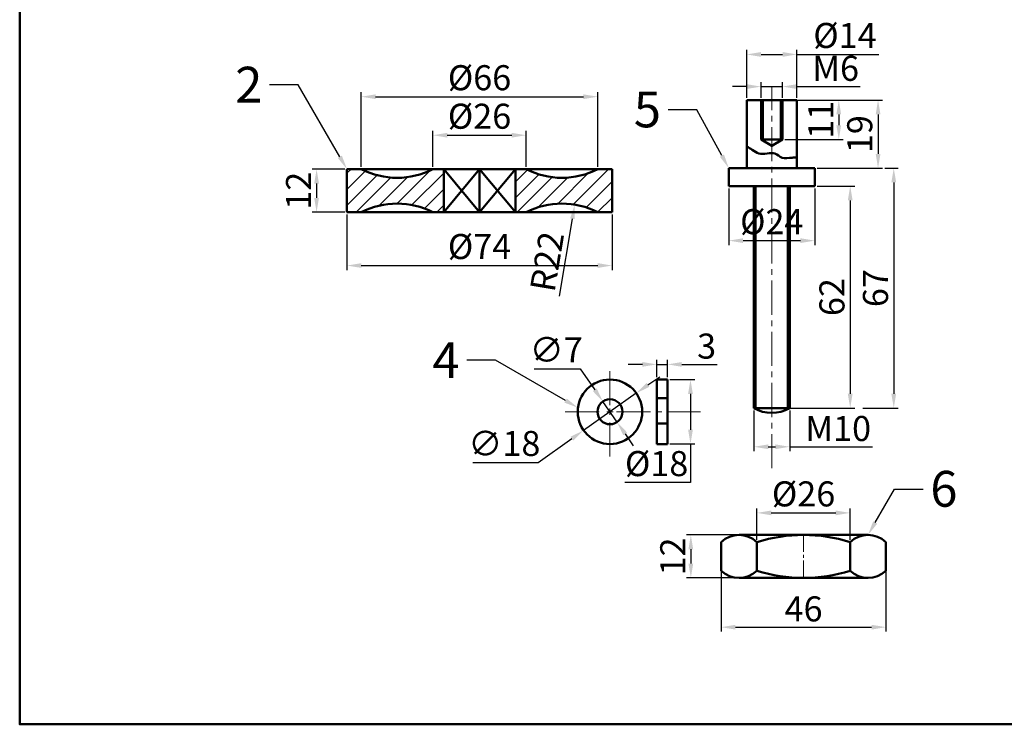
# Model space of a CAD drawing. Units: millimetres. Extents: x 376 to 1043, y -28 to 427.
# Tile 1 of 5: x 376 to 651, y -28 to 168. Entities that reach past the tile are written whole.
import ezdxf
from ezdxf import colors
from ezdxf.entities.mleader import LeaderData, LeaderLine
from ezdxf.math import Vec2, Vec3

# ---------------------------------------------------------------- set-up
doc = ezdxf.new("R2010")
doc.units = ezdxf.units.MM
doc.header["$LTSCALE"] = 0.5
doc.linetypes.add('CENTER2', pattern=[28.575, 19.05, -3.175, 3.175, -3.175])
for name, color, linetype, lineweight in [('M-CNTR', 1, 'CENTER2', 18), ('M-DIMS', 2, 'Continuous', 25), ('M-HATC', 8, 'Continuous', 18), ('M-OUTL', 7, 'Continuous', 50)]:
    doc.layers.add(name, color=color, linetype=linetype, lineweight=lineweight)
doc.styles.get("Standard").update_dxf_attribs({"font": 'arial.ttf'})
doc.dimstyles.new('ISO-25', dxfattribs={"dimtxt": 7, "dimasz": 4, "dimexe": 1.25, "dimexo": 0.625, "dimtad": 1, "dimtoh": 1, "dimtxsty": 'Standard', "dimcen": 2.5, "dimadec": 0, "dimazin": 0, "dimtfac": 1, "dimtmove": 0, "dimatfit": 3, "dimfxl": 1, "dimarcsym": 0})

# ---------------------------------------------------------------- blocks, each defined once
blk = doc.blocks.new('*U4')
at = {"layer": 'M-CNTR', "color": 0, "transparency": 16777216}
for p, q in [((0, 1.8), (0, 12.5)), ((-12.5, 0), (-1.8, 0)), ((1.8, 0), (25.3, 0)), ((0, -12.5), (0, -1.8))]:
    blk.add_line(p, q, dxfattribs=at)
at = {"layer": 'M-CNTR', "color": 0, "linetype": 'Continuous', "transparency": 16777216}
for p, q in [((-0.9, 0), (0.9, 0)), ((0, -0.9), (0, 0.9))]:
    blk.add_line(p, q, dxfattribs=at)
blk = doc.blocks.new('*D5')
at = {"layer": 'Defpoints', "color": 0, "transparency": 16777216}
for p in [(557.3, 72.13), (554.3, 67.9), (557.3, 67.9)]:
    blk.add_point(p, dxfattribs=at)
at = {"layer": 'M-DIMS', "color": 0, "lineweight": -2, "transparency": 16777216}
for p, q in [((550.3, 72.13), (546.3, 72.13)), ((554.3, 68.52), (554.3, 73.38)), ((554.3, 72.13), (557.3, 72.13)), ((557.3, 68.52), (557.3, 73.38)), ((561.3, 72.13), (571.14, 72.13))]:
    blk.add_line(p, q, dxfattribs=at)
at = {"layer": 'M-DIMS', "color": 0, "transparency": 16777216}
for points in [[(550.3, 72.79), (550.3, 71.46), (554.3, 72.13)], [(561.3, 72.79), (561.3, 71.46), (557.3, 72.13)]]:
    blk.add_solid(points, dxfattribs=at)
at = {"layer": 'M-DIMS', "color": 0, "transparency": 16777216, "insert": (568.22, 76.33), "char_height": 7, "attachment_point": 5}
blk.add_mtext('3', dxfattribs=at)
blk = doc.blocks.new('*D6')
at = {"layer": 'Defpoints', "color": 0, "transparency": 16777216}
for p in [(557.3, 67.9), (557.3, 49.9), (563.72, 49.9)]:
    blk.add_point(p, dxfattribs=at)
at = {"layer": 'M-DIMS', "color": 0, "lineweight": -2, "transparency": 16777216}
for p, q in [((557.93, 67.9), (564.97, 67.9)), ((563.72, 63.9), (563.72, 53.9)), ((557.93, 49.9), (564.97, 49.9)), ((563.72, 49.9), (563.72, 39.13)), ((563.72, 39.13), (545.43, 39.13))]:
    blk.add_line(p, q, dxfattribs=at)
at = {"layer": 'M-DIMS', "color": 0, "transparency": 16777216}
for points in [[(563.05, 63.9), (564.38, 63.9), (563.72, 67.9)], [(563.05, 53.9), (564.38, 53.9), (563.72, 49.9)]]:
    blk.add_solid(points, dxfattribs=at)
at = {"layer": 'M-DIMS', "color": 0, "transparency": 16777216, "insert": (554.26, 43.52), "char_height": 7, "attachment_point": 5}
blk.add_mtext('%%C18', dxfattribs=at)
blk = doc.blocks.new('*D7')
at = {"layer": 'Defpoints', "color": 0, "transparency": 16777216}
for p in [(539.25, 61.78), (543.22, 56.01)]:
    blk.add_point(p, dxfattribs=at)
at = {"layer": 'M-DIMS', "color": 0, "lineweight": -2, "transparency": 16777216}
for p, q in [((520.12, 70.91), (532.95, 70.91)), ((532.95, 70.91), (536.98, 65.07)), ((543.22, 56.01), (539.25, 61.78)), ((545.49, 52.72), (547.76, 49.43))]:
    blk.add_line(p, q, dxfattribs=at)
at = {"layer": 'M-DIMS', "color": 0, "transparency": 16777216}
for points in [[(537.53, 65.45), (536.43, 64.69), (539.25, 61.78)], [(546.04, 53.1), (544.94, 52.34), (543.22, 56.01)]]:
    blk.add_solid(points, dxfattribs=at)
at = {"layer": 'M-DIMS', "color": 0, "transparency": 16777216, "insert": (526.23, 75.31), "char_height": 7, "attachment_point": 5}
blk.add_mtext('∅7', dxfattribs=at)
blk = doc.blocks.new('*D8')
at = {"layer": 'Defpoints', "color": 0, "transparency": 16777216}
for p in [(548.59, 64.09), (533.88, 53.7)]:
    blk.add_point(p, dxfattribs=at)
at = {"layer": 'M-DIMS', "color": 0, "lineweight": -2, "transparency": 16777216}
for p, q in [((551.85, 66.4), (555.12, 68.7)), ((548.59, 64.09), (533.88, 53.7)), ((521.19, 44.74), (530.62, 51.4)), ((502.91, 44.74), (521.19, 44.74))]:
    blk.add_line(p, q, dxfattribs=at)
at = {"layer": 'M-DIMS', "color": 0, "transparency": 16777216}
for points in [[(551.47, 66.94), (552.24, 65.85), (548.59, 64.09)], [(530.23, 51.94), (531, 50.85), (533.88, 53.7)]]:
    blk.add_solid(points, dxfattribs=at)
at = {"layer": 'M-DIMS', "color": 0, "transparency": 16777216, "insert": (511.74, 49.13), "char_height": 7, "attachment_point": 5}
blk.add_mtext('∅18', dxfattribs=at)
blk = doc.blocks.new('*D9')
at = {"layer": 'Defpoints', "color": 0, "transparency": 16777216}
for p in [(467.82, 114.63), (541.82, 114.63), (541.82, 99.73)]:
    blk.add_point(p, dxfattribs=at)
at = {"layer": 'M-DIMS', "color": 0, "lineweight": -2, "transparency": 16777216}
for p, q in [((467.82, 114.01), (467.82, 98.48)), ((541.82, 114.01), (541.82, 98.48)), ((471.82, 99.73), (537.82, 99.73))]:
    blk.add_line(p, q, dxfattribs=at)
at = {"layer": 'M-DIMS', "color": 0, "transparency": 16777216}
for points in [[(471.82, 100.4), (471.82, 99.07), (467.82, 99.73)], [(537.82, 100.4), (537.82, 99.07), (541.82, 99.73)]]:
    blk.add_solid(points, dxfattribs=at)
at = {"layer": 'M-DIMS', "color": 0, "transparency": 16777216, "insert": (504.82, 104.13), "char_height": 7, "attachment_point": 5}
blk.add_mtext('%%C74', dxfattribs=at)
blk = doc.blocks.new('*D10')
at = {"layer": 'Defpoints', "color": 0, "transparency": 16777216}
for p in [(537.82, 146.88), (471.82, 126.63), (537.82, 126.63)]:
    blk.add_point(p, dxfattribs=at)
at = {"layer": 'M-DIMS', "color": 0, "lineweight": -2, "transparency": 16777216}
for p, q in [((471.82, 127.26), (471.82, 148.13)), ((475.82, 146.88), (533.82, 146.88)), ((537.82, 127.26), (537.82, 148.13))]:
    blk.add_line(p, q, dxfattribs=at)
at = {"layer": 'M-DIMS', "color": 0, "transparency": 16777216}
for points in [[(475.82, 147.54), (475.82, 146.21), (471.82, 146.88)], [(533.82, 147.54), (533.82, 146.21), (537.82, 146.88)]]:
    blk.add_solid(points, dxfattribs=at)
at = {"layer": 'M-DIMS', "color": 0, "transparency": 16777216, "insert": (504.82, 151.27), "char_height": 7, "attachment_point": 5}
blk.add_mtext('%%C66', dxfattribs=at)
blk = doc.blocks.new('*D11')
at = {"layer": 'Defpoints', "color": 0, "transparency": 16777216}
for p in [(517.82, 136.12), (491.82, 126.63), (517.82, 126.63)]:
    blk.add_point(p, dxfattribs=at)
at = {"layer": 'M-DIMS', "color": 0, "lineweight": -2, "transparency": 16777216}
for p, q in [((491.82, 127.26), (491.82, 137.37)), ((495.82, 136.12), (513.82, 136.12)), ((517.82, 127.26), (517.82, 137.37))]:
    blk.add_line(p, q, dxfattribs=at)
at = {"layer": 'M-DIMS', "color": 0, "transparency": 16777216}
for points in [[(495.82, 136.79), (495.82, 135.46), (491.82, 136.12)], [(513.82, 136.79), (513.82, 135.46), (517.82, 136.12)]]:
    blk.add_solid(points, dxfattribs=at)
at = {"layer": 'M-DIMS', "color": 0, "transparency": 16777216, "insert": (504.82, 140.52), "char_height": 7, "attachment_point": 5}
blk.add_mtext('%%C26', dxfattribs=at)
blk = doc.blocks.new('*D12')
at = {"layer": 'Defpoints', "color": 0, "transparency": 16777216}
for p in [(467.82, 126.63), (459.34, 114.63), (467.82, 114.63)]:
    blk.add_point(p, dxfattribs=at)
at = {"layer": 'M-DIMS', "color": 0, "lineweight": -2, "transparency": 16777216}
for p, q in [((467.2, 126.63), (458.09, 126.63)), ((459.34, 122.63), (459.34, 118.63)), ((467.2, 114.63), (458.09, 114.63))]:
    blk.add_line(p, q, dxfattribs=at)
at = {"layer": 'M-DIMS', "color": 0, "transparency": 16777216}
for points in [[(458.67, 122.63), (460, 122.63), (459.34, 126.63)], [(458.67, 118.63), (460, 118.63), (459.34, 114.63)]]:
    blk.add_solid(points, dxfattribs=at)
at = {"layer": 'M-DIMS', "color": 0, "transparency": 16777216, "insert": (455.2, 120.63), "char_height": 7, "attachment_point": 5, "rotation": 90}
blk.add_mtext('12', dxfattribs=at)
blk = doc.blocks.new('*D13')
at = {"layer": 'Defpoints', "color": 0, "transparency": 16777216}
for p in [(531.42, 116.74), (527.82, 95.04)]:
    blk.add_point(p, dxfattribs=at)
at = {"layer": 'M-DIMS', "color": 0, "lineweight": -2, "transparency": 16777216}
blk.add_line((527.18, 91.18), (530.77, 112.79), dxfattribs=at)
at = {"layer": 'M-DIMS', "color": 0, "transparency": 16777216}
blk.add_solid([(530.11, 112.9), (531.42, 112.68), (531.42, 116.74)], dxfattribs=at)
at = {"layer": 'M-DIMS', "color": 0, "transparency": 16777216, "insert": (524.56, 100.69), "char_height": 7, "attachment_point": 5, "rotation": 80.5866}
blk.add_mtext('R22', dxfattribs=at)
blk = doc.blocks.new('*U14')
at = {"layer": 'M-CNTR', "color": 0, "transparency": 16777216}
blk.add_line((0, -93.3), (0, 13), dxfattribs=at)
blk = doc.blocks.new('*D15')
at = {"layer": 'Defpoints', "color": 0, "transparency": 16777216}
for p in [(589.41, 145.92), (589.41, 134.92), (605.12, 134.92)]:
    blk.add_point(p, dxfattribs=at)
at = {"layer": 'M-DIMS', "color": 0, "lineweight": -2, "transparency": 16777216}
for p, q in [((590.04, 145.92), (606.37, 145.92)), ((605.12, 141.92), (605.12, 138.92)), ((590.04, 134.92), (606.37, 134.92))]:
    blk.add_line(p, q, dxfattribs=at)
at = {"layer": 'M-DIMS', "color": 0, "transparency": 16777216}
for points in [[(604.45, 141.92), (605.78, 141.92), (605.12, 145.92)], [(604.45, 138.92), (605.78, 138.92), (605.12, 134.92)]]:
    blk.add_solid(points, dxfattribs=at)
at = {"layer": 'M-DIMS', "color": 0, "transparency": 16777216, "insert": (600.98, 140.42), "char_height": 7, "attachment_point": 5, "rotation": 90}
blk.add_mtext('11', dxfattribs=at)
blk = doc.blocks.new('*D16')
at = {"layer": 'Defpoints', "color": 0, "transparency": 16777216}
for p in [(593.41, 145.92), (598.41, 126.92), (616.08, 126.92)]:
    blk.add_point(p, dxfattribs=at)
at = {"layer": 'M-DIMS', "color": 0, "lineweight": -2, "transparency": 16777216}
for p, q in [((594.04, 145.92), (617.33, 145.92)), ((616.08, 141.92), (616.08, 130.92)), ((599.04, 126.92), (617.33, 126.92))]:
    blk.add_line(p, q, dxfattribs=at)
at = {"layer": 'M-DIMS', "color": 0, "transparency": 16777216}
for points in [[(615.42, 141.92), (616.75, 141.92), (616.08, 145.92)], [(615.42, 130.92), (616.75, 130.92), (616.08, 126.92)]]:
    blk.add_solid(points, dxfattribs=at)
at = {"layer": 'M-DIMS', "color": 0, "transparency": 16777216, "insert": (611.88, 136.42), "char_height": 7, "attachment_point": 5, "rotation": 90}
blk.add_mtext('19', dxfattribs=at)
blk = doc.blocks.new('*D17')
at = {"layer": 'Defpoints', "color": 0, "transparency": 16777216}
for p in [(598.41, 121.92), (588.21, 59.92), (608.31, 59.92)]:
    blk.add_point(p, dxfattribs=at)
at = {"layer": 'M-DIMS', "color": 0, "lineweight": -2, "transparency": 16777216}
for p, q in [((599.04, 121.92), (609.56, 121.92)), ((608.31, 117.92), (608.31, 63.92)), ((588.83, 59.92), (609.56, 59.92))]:
    blk.add_line(p, q, dxfattribs=at)
at = {"layer": 'M-DIMS', "color": 0, "transparency": 16777216}
for points in [[(607.64, 117.92), (608.98, 117.92), (608.31, 121.92)], [(607.64, 63.92), (608.98, 63.92), (608.31, 59.92)]]:
    blk.add_solid(points, dxfattribs=at)
at = {"layer": 'M-DIMS', "color": 0, "transparency": 16777216, "insert": (604.11, 90.92), "char_height": 7, "attachment_point": 5, "rotation": 90}
blk.add_mtext('62', dxfattribs=at)
blk = doc.blocks.new('*D18')
at = {"layer": 'Defpoints', "color": 0, "transparency": 16777216}
for p in [(589.41, 149.7), (583.41, 145.92), (589.41, 145.92)]:
    blk.add_point(p, dxfattribs=at)
at = {"layer": 'M-DIMS', "color": 0, "lineweight": -2, "transparency": 16777216}
for p, q in [((579.41, 149.7), (575.41, 149.7)), ((583.41, 146.54), (583.41, 150.95)), ((583.41, 149.7), (589.41, 149.7)), ((589.41, 146.54), (589.41, 150.95)), ((593.41, 149.7), (611.07, 149.7))]:
    blk.add_line(p, q, dxfattribs=at)
at = {"layer": 'M-DIMS', "color": 0, "transparency": 16777216}
for points in [[(579.41, 150.37), (579.41, 149.04), (583.41, 149.7)], [(593.41, 150.37), (593.41, 149.04), (589.41, 149.7)]]:
    blk.add_solid(points, dxfattribs=at)
at = {"layer": 'M-DIMS', "color": 0, "transparency": 16777216, "insert": (604.24, 153.9), "char_height": 7, "attachment_point": 5}
blk.add_mtext('M6', dxfattribs=at)
blk = doc.blocks.new('*D19')
at = {"layer": 'Defpoints', "color": 0, "transparency": 16777216}
for p in [(593.41, 158.68), (579.41, 145.92), (593.41, 145.92)]:
    blk.add_point(p, dxfattribs=at)
at = {"layer": 'M-DIMS', "color": 0, "lineweight": -2, "transparency": 16777216}
for p, q in [((579.41, 146.54), (579.41, 159.93)), ((593.41, 146.54), (593.41, 159.93)), ((583.41, 158.68), (589.41, 158.68)), ((593.41, 158.68), (616.28, 158.68))]:
    blk.add_line(p, q, dxfattribs=at)
at = {"layer": 'M-DIMS', "color": 0, "transparency": 16777216}
for points in [[(583.41, 159.35), (583.41, 158.01), (579.41, 158.68)], [(589.41, 159.35), (589.41, 158.01), (593.41, 158.68)]]:
    blk.add_solid(points, dxfattribs=at)
at = {"layer": 'M-DIMS', "color": 0, "transparency": 16777216, "insert": (606.84, 163.07), "char_height": 7, "attachment_point": 5}
blk.add_mtext('%%C14', dxfattribs=at)
blk = doc.blocks.new('*D21')
at = {"layer": 'Defpoints', "color": 0, "transparency": 16777216}
for p in [(574.41, 121.92), (598.41, 121.92), (598.41, 106.68)]:
    blk.add_point(p, dxfattribs=at)
at = {"layer": 'M-DIMS', "color": 0, "lineweight": -2, "transparency": 16777216}
for p, q in [((574.41, 121.29), (574.41, 105.43)), ((598.41, 121.29), (598.41, 105.43)), ((578.41, 106.68), (594.41, 106.68))]:
    blk.add_line(p, q, dxfattribs=at)
at = {"layer": 'M-DIMS', "color": 0, "transparency": 16777216}
for points in [[(578.41, 107.35), (578.41, 106.02), (574.41, 106.68)], [(594.41, 107.35), (594.41, 106.02), (598.41, 106.68)]]:
    blk.add_solid(points, dxfattribs=at)
at = {"layer": 'M-DIMS', "color": 0, "transparency": 16777216, "insert": (586.41, 111.08), "char_height": 7, "attachment_point": 5}
blk.add_mtext('%%C24', dxfattribs=at)
blk = doc.blocks.new('*D22')
at = {"layer": 'Defpoints', "color": 0, "transparency": 16777216}
for p in [(581.41, 59.92), (591.41, 59.92), (591.41, 49.12)]:
    blk.add_point(p, dxfattribs=at)
at = {"layer": 'M-DIMS', "color": 0, "lineweight": -2, "transparency": 16777216}
for p, q in [((581.41, 59.29), (581.41, 47.87)), ((591.41, 59.29), (591.41, 47.87)), ((585.41, 49.12), (587.41, 49.12)), ((591.41, 49.12), (614.49, 49.12))]:
    blk.add_line(p, q, dxfattribs=at)
at = {"layer": 'M-DIMS', "color": 0, "transparency": 16777216}
for points in [[(585.41, 49.79), (585.41, 48.46), (581.41, 49.12)], [(587.41, 49.79), (587.41, 48.46), (591.41, 49.12)]]:
    blk.add_solid(points, dxfattribs=at)
at = {"layer": 'M-DIMS', "color": 0, "transparency": 16777216, "insert": (604.95, 53.32), "char_height": 7, "attachment_point": 5}
blk.add_mtext('M10', dxfattribs=at)
blk = doc.blocks.new('*D23')
at = {"layer": 'Defpoints', "color": 0, "transparency": 16777216}
for p in [(617.33, 126.92), (611.19, 59.92), (620.47, 59.92)]:
    blk.add_point(p, dxfattribs=at)
at = {"layer": 'M-DIMS', "color": 0, "lineweight": -2, "transparency": 16777216}
for p, q in [((617.96, 126.92), (621.72, 126.92)), ((620.47, 122.92), (620.47, 63.92)), ((611.81, 59.92), (621.72, 59.92))]:
    blk.add_line(p, q, dxfattribs=at)
at = {"layer": 'M-DIMS', "color": 0, "transparency": 16777216}
for points in [[(619.8, 122.92), (621.14, 122.92), (620.47, 126.92)], [(619.8, 63.92), (621.14, 63.92), (620.47, 59.92)]]:
    blk.add_solid(points, dxfattribs=at)
at = {"layer": 'M-DIMS', "color": 0, "transparency": 16777216, "insert": (616.27, 93.42), "char_height": 7, "attachment_point": 5, "rotation": 90}
blk.add_mtext('67', dxfattribs=at)
blk = doc.blocks.new('*D54')
at = {"layer": 'Defpoints', "color": 0, "ltscale": 0.5, "transparency": 16777216}
for p in [(572.28, 18.5), (618.28, 18.5), (618.28, -1.25)]:
    blk.add_point(p, dxfattribs=at)
at = {"layer": 'M-DIMS', "color": 0, "lineweight": -2, "ltscale": 0.5, "transparency": 16777216}
for p, q in [((572.28, 17.88), (572.28, -2.5)), ((618.28, 17.88), (618.28, -2.5)), ((576.28, -1.25), (614.28, -1.25))]:
    blk.add_line(p, q, dxfattribs=at)
at = {"layer": 'M-DIMS', "color": 0, "ltscale": 0.5, "transparency": 16777216}
for points in [[(576.28, -0.59), (576.28, -1.92), (572.28, -1.25)], [(614.28, -0.59), (614.28, -1.92), (618.28, -1.25)]]:
    blk.add_solid(points, dxfattribs=at)
at = {"layer": 'M-DIMS', "color": 0, "ltscale": 0.5, "transparency": 16777216, "insert": (595.28, 2.95), "char_height": 7, "attachment_point": 5}
blk.add_mtext('46', dxfattribs=at)
blk = doc.blocks.new('*D55')
at = {"layer": 'Defpoints', "color": 0, "ltscale": 0.5, "transparency": 16777216}
for p in [(577.28, 24.5), (563.82, 12.5), (577.28, 12.5)]:
    blk.add_point(p, dxfattribs=at)
at = {"layer": 'M-DIMS', "color": 0, "lineweight": -2, "ltscale": 0.5, "transparency": 16777216}
for p, q in [((576.66, 24.5), (562.57, 24.5)), ((563.82, 20.5), (563.82, 16.5)), ((576.66, 12.5), (562.57, 12.5))]:
    blk.add_line(p, q, dxfattribs=at)
at = {"layer": 'M-DIMS', "color": 0, "ltscale": 0.5, "transparency": 16777216}
for points in [[(563.15, 20.5), (564.48, 20.5), (563.82, 24.5)], [(563.15, 16.5), (564.48, 16.5), (563.82, 12.5)]]:
    blk.add_solid(points, dxfattribs=at)
at = {"layer": 'M-DIMS', "color": 0, "ltscale": 0.5, "transparency": 16777216, "insert": (559.68, 18.5), "char_height": 7, "attachment_point": 5, "rotation": 90}
blk.add_mtext('12', dxfattribs=at)
blk = doc.blocks.new('*D56')
at = {"layer": 'Defpoints', "color": 0, "ltscale": 0.5, "transparency": 16777216}
for p in [(608.28, 30.66), (582.28, 22.5), (608.28, 22.5)]:
    blk.add_point(p, dxfattribs=at)
at = {"layer": 'M-DIMS', "color": 0, "lineweight": -2, "ltscale": 0.5, "transparency": 16777216}
for p, q in [((582.28, 23.13), (582.28, 31.91)), ((586.28, 30.66), (604.28, 30.66)), ((608.28, 23.13), (608.28, 31.91))]:
    blk.add_line(p, q, dxfattribs=at)
at = {"layer": 'M-DIMS', "color": 0, "ltscale": 0.5, "transparency": 16777216}
for points in [[(586.28, 31.33), (586.28, 30), (582.28, 30.66)], [(604.28, 31.33), (604.28, 30), (608.28, 30.66)]]:
    blk.add_solid(points, dxfattribs=at)
at = {"layer": 'M-DIMS', "color": 0, "ltscale": 0.5, "transparency": 16777216, "insert": (595.28, 35.06), "char_height": 7, "attachment_point": 5}
blk.add_mtext('%%C26', dxfattribs=at)

msp = doc.modelspace()

# ---------------------------------------------------------------- hatches: boundary and pattern name
at = {"layer": 'M-HATC'}
h = msp.add_hatch(dxfattribs=at)
h.set_pattern_fill('ANSI31', color=256)
h.set_pattern_definition([(45, (137.644, -132.84), (-2.245064, 2.245064), [])])
h.paths.add_polyline_path([(467.822, 114.632), (471.822, 114.632, -0.2404082), (491.822, 114.632), (494.822, 114.632), (494.822, 126.632), (491.822, 126.632, -0.2404082), (471.822, 126.632), (467.822, 126.632)])
h.paths.add_polyline_path([(537.822, 114.632), (541.822, 114.632), (541.822, 126.632), (537.822, 126.632, -0.2404082), (517.822, 126.632), (514.822, 126.632), (514.822, 114.632), (517.822, 114.632, -0.2404082)])

# ---------------------------------------------------------------- linework, layer by layer
at = {"layer": 'M-CNTR', "ltscale": 0.5}
msp.add_line((595.28, 24.504), (595.28, 12.504), dxfattribs=at)
at = {"layer": 'M-OUTL'}
for p, q in [((579.412, 145.92), (593.412, 145.92)), ((579.412, 126.92), (579.412, 145.92)), ((583.412, 145.92), (583.412, 134.92)), ((583.912, 145.92), (583.912, 134.92)), ((588.912, 145.92), (588.912, 134.92)), ((589.412, 145.92), (589.412, 134.92)), ((593.412, 145.92), (593.412, 126.92)), ((583.412, 134.92), (589.412, 134.92)), ((583.412, 134.92), (586.412, 133.188)), ((586.412, 133.188), (589.412, 134.92)), ((541.822, 126.632), (467.822, 126.632)), ((467.822, 126.632), (467.822, 114.632)), ((494.822, 126.632), (494.822, 114.632)), ((494.822, 114.632), (504.822, 126.632)), ((494.822, 126.632), (504.822, 114.632)), ((504.822, 126.632), (504.822, 114.632)), ((504.822, 126.632), (514.822, 114.632)), ((504.822, 114.632), (514.822, 126.632)), ((514.822, 126.632), (514.822, 114.632)), ((541.822, 114.632), (541.822, 126.632)), ((574.412, 121.92), (574.412, 126.92)), ((574.412, 126.92), (579.412, 126.92)), ((593.412, 126.92), (579.412, 126.92)), ((593.412, 126.92), (598.412, 126.92)), ((598.412, 126.92), (598.412, 121.92)), ((598.412, 121.92), (574.412, 121.92)), ((581.412, 121.92), (581.412, 59.92)), ((581.912, 121.92), (581.912, 59.92)), ((590.912, 121.92), (590.912, 59.92)), ((591.412, 121.92), (591.412, 59.92)), ((467.822, 114.632), (541.822, 114.632)), ((554.303, 67.897), (554.303, 49.897)), ((557.303, 67.897), (554.303, 67.897)), ((557.303, 49.897), (557.303, 67.897)), ((554.303, 62.702), (557.303, 62.702)), ((581.412, 59.92), (591.412, 59.92)), ((554.303, 55.639), (557.303, 55.639)), ((554.303, 49.897), (557.303, 49.897))]:
    msp.add_line(p, q, dxfattribs=at)
at = {"layer": 'M-OUTL', "ltscale": 0.5}
for p, q in [((572.28, 22.504), (572.28, 14.504)), ((613.28, 24.504), (577.28, 24.504)), ((582.28, 22.504), (582.28, 14.504)), ((608.28, 22.504), (608.28, 14.504)), ((618.28, 14.504), (618.28, 22.504)), ((577.28, 12.504), (613.28, 12.504))]:
    msp.add_line(p, q, dxfattribs=at)
msp.add_lwpolyline([(376.448, 426.986), (1042.916, 426.986), (1042.916, -28.377), (376.448, -28.377)], close=True, dxfattribs=at)
at = {"layer": 'M-OUTL'}
for radius in [9, 3.5]:
    msp.add_circle((541.234, 58.897), radius, dxfattribs=at)
for centre, radius, start, end in [((481.822, 146.227), 22, 242.96431, 297.03569), ((527.822, 146.227), 22, 242.96431, 297.03569), ((481.822, 95.036), 22, 62.96431, 117.03569), ((527.822, 95.036), 22, 62.96431, 117.03569), ((586.412, 68.58), 10, 240, 300)]:
    msp.add_arc(centre, radius, start, end, dxfattribs=at)
at = {"layer": 'M-OUTL', "ltscale": 0.5}
for centre, radius, start, end in [((577.28, 17.254), 7.25, 46.39718, 133.60282), ((595.28, -18.746), 43.25, 72.50768, 107.49232), ((613.28, 17.254), 7.25, 46.39718, 133.60282), ((577.28, 19.754), 7.25, 226.39718, 313.60282), ((595.28, 55.754), 43.25, 252.50768, 287.49232), ((613.28, 19.754), 7.25, 226.39718, 313.60282)]:
    msp.add_arc(centre, radius, start, end, dxfattribs=at)
at = {"layer": 'M-OUTL'}
msp.add_open_spline([(579.412, 132.96), (579.925, 132.683), (581.063, 132.069), (582.77, 130.697), (585.06, 130.985), (587.432, 131.371), (589.311, 129.33), (591.61, 129.912), (592.972, 129.867), (593.412, 129.852)], degree=3, knots=[0, 0, 0, 0, 1.7625401, 3.9066768, 6.2232346, 8.4032096, 10.7123205, 13.4999601, 14.8327576, 14.8327576, 14.8327576, 14.8327576], dxfattribs=at)

# ---------------------------------------------------------------- block references
at = {"layer": 'M-CNTR'}
for name, p in [('*U14', (586.412, 136.42)), ('*U4', (541.234, 58.897))]:
    msp.add_blockref(name, p, dxfattribs=at)

# ---------------------------------------------------------------- dimensions: what is measured, and where the dimension line sits
at = {"layer": 'M-DIMS'}
for base, p1, p2, text, picture, middle in [((593.412, 158.679), (579.412, 145.92), (593.412, 145.92), '%%C<>', '*D19', (606.844, 163.074)), ((589.412, 149.705), (583.412, 145.92), (589.412, 145.92), 'M<>', '*D18', (604.242, 153.904)), ((541.822, 99.733), (467.822, 114.632), (541.822, 114.632), '%%C<>', '*D9', (504.822, 104.128)), ((591.412, 49.123), (581.412, 59.92), (591.412, 59.92), 'M<>', '*D22', (604.952, 53.322))]:
    dim = msp.add_linear_dim(base=base, p1=p1, p2=p2, text=text, dimstyle='ISO-25', override={"dimclrd": 0, "dimclre": 0, "dimclrt": 0}, dxfattribs=at)
    dim.commit()
    dim.dimension.update_dxf_attribs({"geometry": picture, "text_midpoint": middle})
for base, p1, p2, picture, middle in [((537.822, 146.877), (471.822, 126.632), (537.822, 126.632), '*D10', (504.822, 146.877)), ((517.822, 136.122), (491.822, 126.632), (517.822, 126.632), '*D11', (504.822, 136.122)), ((598.412, 106.685), (574.412, 121.92), (598.412, 121.92), '*D21', (586.412, 106.685))]:
    dim = msp.add_linear_dim(base=base, p1=p1, p2=p2, text='%%C<>', dimstyle='ISO-25', override={"dimclrd": 0, "dimclre": 0, "dimclrt": 0}, dxfattribs=at)
    dim.commit()
    dim.dimension.update_dxf_attribs({"geometry": picture, "text_midpoint": middle, "dimtype": 160})
for base, p1, p2, picture, middle in [((605.117, 134.92), (589.412, 145.92), (589.412, 134.92), '*D15', (600.977, 140.42)), ((616.082, 126.92), (593.412, 145.92), (598.412, 126.92), '*D16', (611.883, 136.42)), ((459.338, 114.632), (467.822, 126.632), (467.822, 114.632), '*D12', (455.199, 120.632))]:
    dim = msp.add_linear_dim(base=base, p1=p1, p2=p2, angle=90, dimstyle='ISO-25', override={"dimclrd": 0, "dimclre": 0, "dimclrt": 0}, dxfattribs=at)
    dim.commit()
    dim.dimension.update_dxf_attribs({"geometry": picture, "text_midpoint": middle})
for base, p1, p2, picture, middle in [((620.469, 59.92), (617.332, 126.92), (611.187, 59.92), '*D23', (620.469, 93.42)), ((608.309, 59.92), (598.412, 121.92), (588.207, 59.92), '*D17', (608.309, 90.92))]:
    dim = msp.add_linear_dim(base=base, p1=p1, p2=p2, angle=90, dimstyle='ISO-25', override={"dimclrd": 0, "dimclre": 0, "dimclrt": 0}, dxfattribs=at)
    dim.commit()
    dim.dimension.update_dxf_attribs({"geometry": picture, "text_midpoint": middle, "dimtype": 160})
dim = msp.add_radius_dim(center=(527.822, 95.036), mpoint=(531.421, 116.739), dimstyle='ISO-25', override={"dimclrd": 0, "dimclre": 0, "dimclrt": 0}, dxfattribs=at)
dim.commit()
dim.dimension.update_dxf_attribs({"geometry": '*D13', "text_midpoint": (528.648, 100.015), "dimtype": 164})
dim = msp.add_diameter_dim_2p(p1=(543.22, 56.015), p2=(539.248, 61.779), dimstyle='ISO-25', override={"dimclrd": 0, "dimclre": 0, "dimclrt": 0}, dxfattribs=at)
dim.commit()
dim.dimension.update_dxf_attribs({"geometry": '*D7', "text_midpoint": (526.226, 70.914), "dimtype": 163})
dim = msp.add_linear_dim(base=(557.303, 72.127), p1=(554.303, 67.897), p2=(557.303, 67.897), dimstyle='ISO-25', override={"dimclrd": 0, "dimclre": 0, "dimclrt": 0}, dxfattribs=at)
dim.commit()
dim.dimension.update_dxf_attribs({"geometry": '*D5', "text_midpoint": (568.22, 76.328)})
dim = msp.add_diameter_dim_2p(p1=(548.586, 64.088), p2=(533.883, 53.705), dimstyle='ISO-25', override={"dimclrd": 0, "dimclre": 0, "dimclrt": 0}, dxfattribs=at)
dim.commit()
dim.dimension.update_dxf_attribs({"geometry": '*D8', "text_midpoint": (511.736, 49.135)})
dim = msp.add_linear_dim(base=(563.718, 49.897), p1=(557.303, 67.897), p2=(557.303, 49.897), angle=90, text='%%C<>', dimstyle='ISO-25', override={"dimclrd": 0, "dimclre": 0, "dimclrt": 0}, dxfattribs=at)
dim.commit()
dim.dimension.update_dxf_attribs({"geometry": '*D6', "text_midpoint": (554.264, 39.127), "dimtype": 160})
at = {"layer": 'M-DIMS', "ltscale": 0.5}
dim = msp.add_linear_dim(base=(608.28, 30.663), p1=(582.28, 22.504), p2=(608.28, 22.504), text='%%C<>', dimstyle='ISO-25', override={"dimclrd": 0, "dimclre": 0, "dimclrt": 0}, dxfattribs=at)
dim.commit()
dim.dimension.update_dxf_attribs({"geometry": '*D56', "text_midpoint": (595.28, 35.057)})
dim = msp.add_linear_dim(base=(563.817, 12.504), p1=(577.28, 24.504), p2=(577.28, 12.504), angle=90, dimstyle='ISO-25', override={"dimclrd": 0, "dimclre": 0, "dimclrt": 0}, dxfattribs=at)
dim.commit()
dim.dimension.update_dxf_attribs({"geometry": '*D55', "text_midpoint": (559.678, 18.504)})
dim = msp.add_linear_dim(base=(618.28, -1.252), p1=(572.28, 18.504), p2=(618.28, 18.504), dimstyle='ISO-25', override={"dimclrd": 0, "dimclre": 0, "dimclrt": 0}, dxfattribs=at)
dim.commit()
dim.dimension.update_dxf_attribs({"geometry": '*D54', "text_midpoint": (595.28, 2.947)})

# ---------------------------------------------------------------- leaders
at = {"layer": 'M-DIMS'}
ml = msp.add_multileader_mtext('Standard', dxfattribs=at)
ml.set_content('2', color=256)
ml.set_leader_properties()
ml.build(insert=Vec2(0, 0))
ctx = ml.context
ctx.base_point, ctx.char_height, ctx.plane_origin = Vec3(435.57, 150.237), 10, Vec3(467.822, 126.632)
ctx.text_align_type = 2
notes = []
notes.append((ctx, [(0, (1, 1, 0), (454.194, 150.237), (-1, 0), 8, [(0, [(467.822, 126.632)], 0, [])])]))
ctx.mtext.insert, ctx.mtext.alignment, ctx.mtext.flow_direction = Vec3(444.194, 155.237), 3, 5
ml = msp.add_multileader_mtext('Standard', dxfattribs=at)
ml.set_content('5', color=256)
ml.set_leader_properties()
ml.build(insert=Vec2(0, 0))
ctx = ml.context
ctx.base_point, ctx.char_height, ctx.plane_origin = Vec3(546.843, 143.242), 10, Vec3(574.412, 127.759)
ctx.text_align_type = 2
notes.append((ctx, [(0, (1, 1, 0), (565.473, 143.242), (-1, 0), 8, [(0, [(574.412, 126.92)], 0, [])])]))
ctx.mtext.insert, ctx.mtext.alignment, ctx.mtext.flow_direction = Vec3(555.473, 148.328), 3, 5
ml = msp.add_multileader_mtext('Standard', dxfattribs=at)
ml.set_content('4', color=256)
ml.set_leader_properties()
ml.build(insert=Vec2(0, 0))
ctx = ml.context
ctx.base_point, ctx.char_height, ctx.plane_origin = Vec3(490.347, 73.331), 10, Vec3(532.306, 60.028)
ctx.text_align_type = 2
notes.append((ctx, [(0, (1, 1, 0), (509.264, 73.331), (-1, 0), 8, [(0, [(532.306, 60.028)], 0, [])])]))
ctx.mtext.insert, ctx.mtext.alignment, ctx.mtext.flow_direction = Vec3(499.264, 78.331), 3, 5
at = {"layer": 'M-DIMS', "ltscale": 0.5}
ml = msp.add_multileader_mtext('Standard', dxfattribs=at)
ml.set_content('6', color=256)
ml.set_leader_properties()
ml.build(insert=Vec2(0, 0))
ctx = ml.context
ctx.base_point, ctx.char_height, ctx.plane_origin = Vec3(628.67, 37.304), 10, Vec3(613.28, 24.504)
notes.append((ctx, [(0, (1, 1, 0), (620.67, 37.304), (1, 0), 8, [(0, [(613.28, 24.504)], 0, [])])]))
ctx.mtext.insert, ctx.mtext.flow_direction = Vec3(630.67, 42.389), 5
for ctx, leaders in notes:
    for number, flags, end, landing, length, lines in leaders:
        leader = LeaderData()
        leader.index, (leader.has_last_leader_line, leader.has_dogleg_vector, leader.attachment_direction) = number, flags
        leader.last_leader_point, leader.dogleg_vector, leader.dogleg_length = Vec3(end), Vec3(landing), length
        for number, points, colour, breaks in lines:
            line = LeaderLine()
            line.index, line.vertices, line.color, line.breaks = number, Vec3.list(points), colors.encode_raw_color(colour), breaks
            leader.lines.append(line)
        ctx.leaders.append(leader)

doc.saveas('drawing.dxf')
